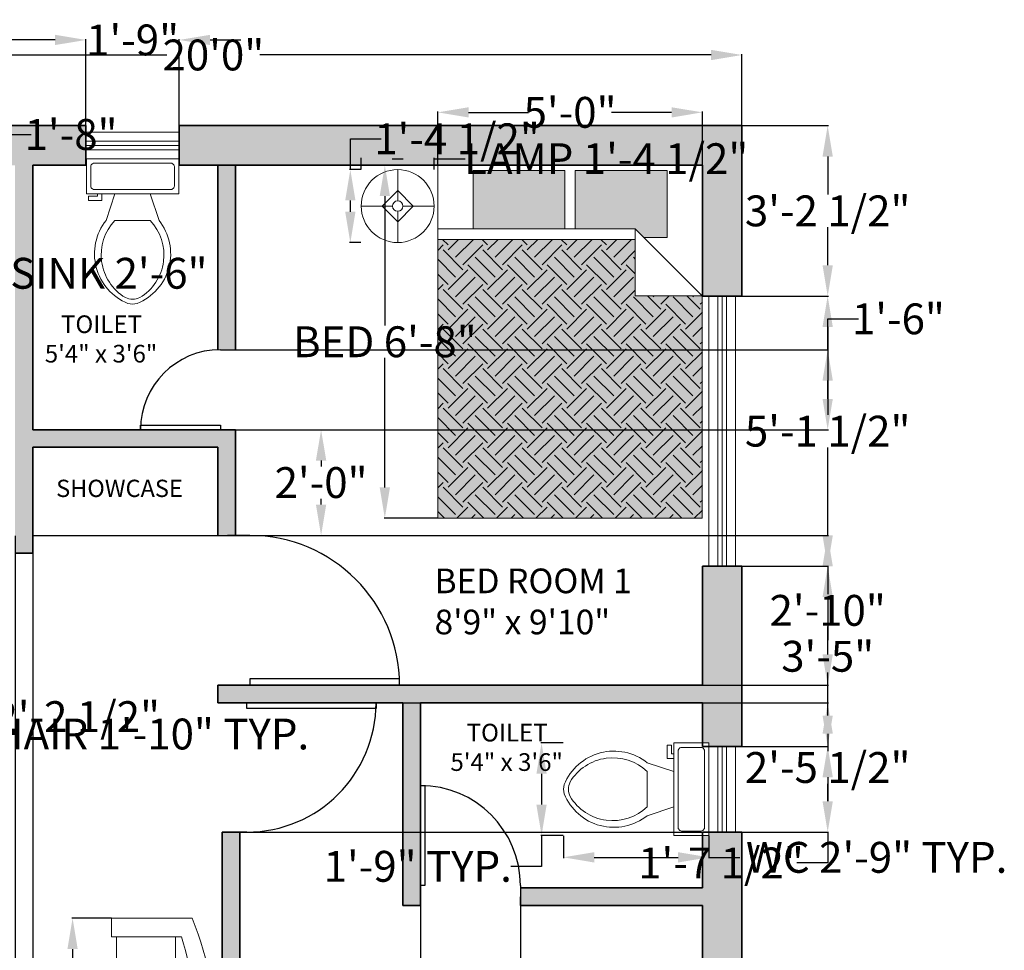
# Model space of a CAD drawing. Units: inches. Extents: x -8 to 329, y 10 to 430.
# Tile 4 of 4: x 106 to 329, y 213 to 424. Entities that reach past the tile are written whole.
import ezdxf

# ---------------------------------------------------------------- set-up
doc = ezdxf.new("R2010")
doc.units = ezdxf.units.IN
doc.header["$MEASUREMENT"] = 0
for name, color, linetype, lineweight in [('A-ANNO-DIMS', 2, 'Continuous', 18), ('A-ANNO-TEXT', 7, 'Continuous', 18), ('A-AREA-IDEN', 7, 'Continuous', 18), ('A-DOOR', 3, 'Continuous', 25), ('A-FLOR-CASE', 9, 'Continuous', 25), ('A-FLOR-FIXT', 9, 'Continuous', 18), ('A-FURN', 8, 'Continuous', 18), ('A-GLAZ', 4, 'Continuous', 18), ('A-WALL', 7, 'Continuous', 35), ('A-WALL-PATT', 253, 'Continuous', 13)]:
    doc.layers.add(name, color=color, linetype=linetype, lineweight=lineweight)
doc.layers.add('A-FURN-BASE-PATT', color=144, linetype='Continuous', lineweight=13, true_color=0x1e788f)
doc.layers.add('A-FURN-PATT', color=39, linetype='Continuous', lineweight=13, true_color=0x603913)
doc.styles.get("Standard").update_dxf_attribs({"font": 'arial.ttf'})
doc.dimstyles.get("Standard").update_dxf_attribs({"dimtxt": 7, "dimasz": 7, "dimexe": 0.18, "dimexo": 0.0625, "dimgap": 0.09, "dimtad": 0, "dimtih": 1, "dimtoh": 1, "dimdec": 0, "dimzin": 0, "dimdsep": 46, "dimlunit": 3, "dimtxsty": 'Standard', "dimcen": 0.09, "dimadec": 0, "dimazin": 0, "dimtfac": 1, "dimtdec": 0, "dimtofl": 0, "dimtmove": 0, "dimatfit": 3, "dimfxl": 1, "dimtolj": 1, "dimtzin": 0, "dimarcsym": 0})
pattern_1 = [(45, (0, 0), (0, 8.98026), [6.35, -6.35]), (45, (-1.684, 1.684), (0, 8.98026), [6.35, -6.35]), (45, (-3.3676, 3.3676), (0, 8.98026), [6.35, -6.35]), (135, (-3.3676, 4.49), (-8.98026, 0), [6.35, -6.35]), (135, (-1.684, 6.174), (-8.98026, 0), [6.35, -6.35]), (135, (0, 7.858), (-8.98026, 0), [6.35, -6.35])]

# ---------------------------------------------------------------- blocks, each defined once
blk = doc.blocks.new('Bed - Queen')
for p, q in [((0, -80.00003), (0, 0)), ((0, 0), (59.99999, 0)), ((59.99999, 0), (59.99999, -80.00003)), ((7.99999, -1.2), (28.79998, -1.2)), ((7.99999, -14.4), (7.99999, -1.2)), ((28.79998, -1.2), (28.79998, -14.4)), ((31.19999, -1.2), (51.99999, -1.2)), ((31.19999, -14.4), (31.19999, -1.2)), ((51.99999, -1.2), (51.99999, -16.4)), ((0, -14.4), (44.8, -14.4)), ((59.99999, -29.6), (44.8, -14.4)), ((44.8, -14.4), (44.8, -29.6)), ((44.8, -16.8), (0, -16.8)), ((51.99999, -16.4), (46.79936, -16.4)), ((44.8, -29.6), (59.99999, -29.6)), ((59.99999, -80.00003), (0, -80.00003))]:
    blk.add_line(p, q)
blk = doc.blocks.new('Sofa - Roundback 7 ft.')
for p, q in [((-12.00002, -32.4421), (-12.00003, -6.5971)), ((11.99997, -32.4421), (11.99998, -6.5971)), ((-36.000027, -34), (-36.000027, -11.4696)), ((35.99998, -34), (35.99998, -11.4696)), ((-35.999844, -13.3819), (35.9998, -13.3819)), ((-36.000027, -32.4421), (35.99998, -32.4421))]:
    blk.add_line(p, q)
for points in [[(-36.000027, -34), (-42.000027, -34), (-42.000027, -8)], [(41.99998, -8), (41.99998, -34), (35.99998, -34)]]:
    blk.add_lwpolyline(points)
for centre, radius, start, end in [((0, -114.25), 114.25, 68.43141, 111.5686), ((-0.00001, -127.1968), 121.1968, 72.72033, 107.2797)]:
    blk.add_arc(centre, radius, start, end)
blk = doc.blocks.new('Toilet - top')
for p, q in [((9.5, -6), (9.5, -2)), ((-10, -8.5), (-8, -8.5)), ((-10, -9.5), (-10, -8.5)), ((-8, -8.5), (-8, -8)), ((-7, -8), (-7, -9.5)), ((-4, -8), (-6, -14)), ((4, -8), (6, -14)), ((-7, -9.5), (-10, -9.5)), ((4, -14), (-4, -14))]:
    blk.add_line(p, q)
blk.add_lwpolyline([(10.5, -8), (10.5, 0), (-10.5, 0), (-10.5, -8)], close=True)
for points in [[(-9.5, -2), (-9.5, -6)], [(8.5, -1), (-8.5, -1)], [(-8.5, -7), (8.5, -7)]]:
    blk.add_lwpolyline(points)
for centre, radius, start, end in [((-8.62, -1.88), 0.884, 81.8699, 188.1301), ((8.62, -1.88), 0.884, 351.8699, 98.1301), ((-8.62, -6.12), 0.884, 171.8699, 278.1301), ((8.62, -6.12), 0.884, 261.8699, 8.1301), ((3.52, -21.58), 12.17, 141.4691, 247.9714), ((4.2, -21.82), 11.33, 136.3677, 238.9468), ((-3.52, -21.58), 12.17, 292.0284, 38.5307), ((-4.2, -21.82), 11.33, 301.053, 43.6321), ((0, -27.88), 4, 245.7318, 294.2682), ((0, -29), 4, 254.8605, 285.1395)]:
    blk.add_arc(centre, radius, start, end)
blk = doc.blocks.new('*U10')
for p, q in [((0, 0), (0, -6)), ((40, 0), (40, -6))]:
    blk.add_line(p, q)
blk.add_lwpolyline([(0, 0), (0, 40), (1.75, 40), (1.75, 0)], close=True)
blk.add_arc((0, 0), 40, 0, 90)
blk = doc.blocks.new('*U13')
for p, q in [((0, 0), (0, -6)), ((32, 0), (32, -6))]:
    blk.add_line(p, q)
blk.add_lwpolyline([(0, 0), (0, 32), (1.75, 32), (1.75, 0)], close=True)
blk.add_arc((0, 0), 32, 0, 90)
blk = doc.blocks.new('*U12')
for p, q in [((0, 0), (0, -6)), ((-40, 0), (-40, -6))]:
    blk.add_line(p, q)
blk.add_lwpolyline([(0, 0), (0, 40), (-1.75, 40), (-1.75, 0)], close=True)
blk.add_arc((0, 0), 40, 90, 180)
blk = doc.blocks.new('Lamp - Table')
for p, q in [((0, 7), (0, 1)), ((0, 3), (-3, 0)), ((3, 0), (0, 3)), ((-1, 0), (-7, 0)), ((-3, 0), (0, -3)), ((0, -3), (3, 0)), ((1, 0), (7, 0)), ((0, -1), (0, -7))]:
    blk.add_line(p, q)
for radius in [7, 1]:
    blk.add_circle((0, 0), radius)
blk = doc.blocks.new('*D16')
at = {"layer": 'A-ANNO-DIMS', "color": 0, "lineweight": -2, "transparency": 16777216}
for p, q in [((29.9, 399.83), (29.9, 415.98)), ((36.9, 415.8), (139.36, 415.8)), ((262.9, 415.8), (160.45, 415.8)), ((269.9, 399.83), (269.9, 415.98))]:
    blk.add_line(p, q, dxfattribs=at)
at = {"layer": 'A-ANNO-DIMS', "color": 0, "transparency": 16777216}
for points in [[(36.9, 416.96), (36.9, 414.63), (29.9, 415.8)], [(262.9, 416.96), (262.9, 414.63), (269.9, 415.8)]]:
    blk.add_solid(points, dxfattribs=at)
at = {"layer": 'Defpoints', "color": 0, "transparency": 16777216}
for p in [(269.9, 415.8), (29.9, 399.76), (269.9, 399.76)]:
    blk.add_point(p, dxfattribs=at)
at = {"layer": 'A-ANNO-DIMS', "color": 0, "transparency": 16777216, "insert": (149.9, 415.8), "char_height": 7, "attachment_point": 5}
blk.add_mtext('\\A1;20\'0"', dxfattribs=at)
blk = doc.blocks.new('*D18')
at = {"layer": 'A-ANNO-DIMS', "color": 0, "lineweight": -2, "transparency": 16777216}
for p, q in [((200.77, 390.76), (188.64, 390.76)), ((188.82, 383.76), (188.82, 354.38)), ((188.82, 317.68), (188.82, 347.06)), ((200.77, 310.68), (188.64, 310.68))]:
    blk.add_line(p, q, dxfattribs=at)
at = {"layer": 'A-ANNO-DIMS', "color": 0, "transparency": 16777216}
for points in [[(187.65, 383.76), (189.99, 383.76), (188.82, 390.76)], [(187.65, 317.68), (189.99, 317.68), (188.82, 310.68)]]:
    blk.add_solid(points, dxfattribs=at)
at = {"layer": 'Defpoints', "color": 0, "transparency": 16777216}
for p in [(188.82, 390.76), (200.83, 390.76), (200.83, 310.68)]:
    blk.add_point(p, dxfattribs=at)
at = {"layer": 'A-ANNO-DIMS', "color": 0, "transparency": 16777216, "insert": (188.82, 350.72), "char_height": 7, "attachment_point": 5}
blk.add_mtext('\\A1;BED 6\'-8"', dxfattribs=at)
blk = doc.blocks.new('*D19')
at = {"layer": 'A-ANNO-DIMS', "color": 0, "lineweight": -2, "transparency": 16777216}
for p, q in [((200.83, 390.83), (200.83, 402.96)), ((207.83, 402.78), (221.47, 402.78)), ((253.9, 402.78), (240.26, 402.78)), ((260.9, 390.83), (260.9, 402.96))]:
    blk.add_line(p, q, dxfattribs=at)
at = {"layer": 'A-ANNO-DIMS', "color": 0, "transparency": 16777216}
for points in [[(207.83, 403.94), (207.83, 401.61), (200.83, 402.78)], [(253.9, 403.94), (253.9, 401.61), (260.9, 402.78)]]:
    blk.add_solid(points, dxfattribs=at)
at = {"layer": 'Defpoints', "color": 0, "transparency": 16777216}
for p in [(260.9, 402.78), (200.83, 390.76), (260.9, 390.76)]:
    blk.add_point(p, dxfattribs=at)
at = {"layer": 'A-ANNO-DIMS', "color": 0, "transparency": 16777216, "insert": (230.87, 402.78), "char_height": 7, "attachment_point": 5}
blk.add_mtext('\\A1;5\'-0"', dxfattribs=at)
blk = doc.blocks.new('*D22')
at = {"layer": 'A-ANNO-DIMS', "color": 0, "lineweight": -2, "transparency": 16777216}
for p, q in [((40.19, 261.77), (40.19, 265.83)), ((47.19, 265.65), (59.46, 265.65)), ((66.46, 261.77), (66.46, 265.83)), ((66.46, 265.65), (73.46, 265.65))]:
    blk.add_line(p, q, dxfattribs=at)
at = {"layer": 'A-ANNO-DIMS', "color": 0, "transparency": 16777216}
for points in [[(47.19, 266.81), (47.19, 264.48), (40.19, 265.65)], [(59.46, 266.81), (59.46, 264.48), (66.46, 265.65)]]:
    blk.add_solid(points, dxfattribs=at)
at = {"layer": 'Defpoints', "color": 0, "transparency": 16777216}
for p in [(66.46, 265.65), (40.19, 261.71), (66.46, 261.71)]:
    blk.add_point(p, dxfattribs=at)
at = {"layer": 'A-ANNO-DIMS', "color": 0, "transparency": 16777216, "insert": (105.53, 265.65), "char_height": 7, "attachment_point": 5}
blk.add_mtext('\\A1;LAMP 2\'-2 1/2"', dxfattribs=at)
blk = doc.blocks.new('*D24')
at = {"layer": 'A-ANNO-DIMS', "color": 0, "lineweight": -2, "transparency": 16777216}
for p, q in [((183.47, 389.84), (183.47, 392.44)), ((190.47, 392.26), (193.02, 392.26)), ((200.02, 389.84), (200.02, 392.44)), ((200.02, 392.26), (207.02, 392.26))]:
    blk.add_line(p, q, dxfattribs=at)
at = {"layer": 'A-ANNO-DIMS', "color": 0, "transparency": 16777216}
for points in [[(190.47, 393.43), (190.47, 391.09), (183.47, 392.26)], [(193.02, 393.43), (193.02, 391.09), (200.02, 392.26)]]:
    blk.add_solid(points, dxfattribs=at)
at = {"layer": 'Defpoints', "color": 0, "transparency": 16777216}
for p in [(200.02, 392.26), (183.47, 389.78), (200.02, 389.78)]:
    blk.add_point(p, dxfattribs=at)
at = {"layer": 'A-ANNO-DIMS', "color": 0, "transparency": 16777216, "insert": (239.08, 392.26), "char_height": 7, "attachment_point": 5}
blk.add_mtext('\\A1;LAMP 1\'-4 1/2"', dxfattribs=at)
blk = doc.blocks.new('*D25')
at = {"layer": 'A-ANNO-DIMS', "color": 0, "lineweight": -2, "transparency": 16777216}
for p, q in [((180.99, 389.78), (180.99, 396.78)), ((180.99, 396.78), (187.99, 396.78)), ((183.41, 389.78), (180.81, 389.78)), ((180.99, 380.23), (180.99, 382.78)), ((183.41, 373.23), (180.81, 373.23))]:
    blk.add_line(p, q, dxfattribs=at)
at = {"layer": 'A-ANNO-DIMS', "color": 0, "transparency": 16777216}
for points in [[(179.82, 382.78), (182.16, 382.78), (180.99, 389.78)], [(179.82, 380.23), (182.16, 380.23), (180.99, 373.23)]]:
    blk.add_solid(points, dxfattribs=at)
at = {"layer": 'Defpoints', "color": 0, "transparency": 16777216}
for p in [(180.99, 389.78), (183.47, 389.78), (183.47, 373.23)]:
    blk.add_point(p, dxfattribs=at)
at = {"layer": 'A-ANNO-DIMS', "color": 0, "transparency": 16777216, "insert": (205.21, 396.78), "char_height": 7, "attachment_point": 5}
blk.add_mtext('\\A1;1\'-4 1/2"', dxfattribs=at)
blk = doc.blocks.new('*D28')
at = {"layer": 'A-ANNO-DIMS', "color": 0, "lineweight": -2, "transparency": 16777216}
for p, q in [((63.23, 258.5), (63.23, 261.88)), ((70.23, 261.7), (78.03, 261.7)), ((85.03, 258.5), (85.03, 261.88)), ((85.03, 261.7), (92.03, 261.7))]:
    blk.add_line(p, q, dxfattribs=at)
at = {"layer": 'A-ANNO-DIMS', "color": 0, "transparency": 16777216}
for points in [[(70.23, 262.87), (70.23, 260.54), (63.23, 261.7)], [(78.03, 262.87), (78.03, 260.54), (85.03, 261.7)]]:
    blk.add_solid(points, dxfattribs=at)
at = {"layer": 'Defpoints', "color": 0, "transparency": 16777216}
for p in [(85.03, 261.7), (63.23, 258.43), (85.03, 258.43)]:
    blk.add_point(p, dxfattribs=at)
at = {"layer": 'A-ANNO-DIMS', "color": 0, "transparency": 16777216, "insert": (132.71, 261.7), "char_height": 7, "attachment_point": 5}
blk.add_mtext('\\A1;CHAIR 1\'-10" TYP.', dxfattribs=at)
blk = doc.blocks.new('*D30')
at = {"layer": 'A-ANNO-DIMS', "color": 0, "lineweight": -2, "transparency": 16777216}
for p, q in [((229.35, 238.6), (229.35, 233.53)), ((262.4, 238.6), (262.4, 233.53)), ((236.35, 233.71), (255.4, 233.71)), ((262.4, 233.71), (269.4, 233.71))]:
    blk.add_line(p, q, dxfattribs=at)
at = {"layer": 'A-ANNO-DIMS', "color": 0, "transparency": 16777216}
for points in [[(236.35, 234.88), (236.35, 232.54), (229.35, 233.71)], [(255.4, 234.88), (255.4, 232.54), (262.4, 233.71)]]:
    blk.add_solid(points, dxfattribs=at)
at = {"layer": 'Defpoints', "color": 0, "transparency": 16777216}
for p in [(229.35, 238.67), (262.4, 238.67), (262.4, 233.71)]:
    blk.add_point(p, dxfattribs=at)
at = {"layer": 'A-ANNO-DIMS', "color": 0, "transparency": 16777216, "insert": (300.47, 233.71), "char_height": 7, "attachment_point": 5}
blk.add_mtext('\\A1;WC 2\'-9" TYP.', dxfattribs=at)
blk = doc.blocks.new('*D31')
at = {"layer": 'A-ANNO-DIMS', "color": 0, "lineweight": -2, "transparency": 16777216}
for p, q in [((229.29, 259.67), (224.22, 259.67)), ((224.4, 252.67), (224.4, 245.67)), ((229.29, 238.67), (224.22, 238.67)), ((224.4, 238.67), (224.4, 231.67)), ((224.4, 231.67), (217.4, 231.67))]:
    blk.add_line(p, q, dxfattribs=at)
at = {"layer": 'A-ANNO-DIMS', "color": 0, "transparency": 16777216}
for points in [[(223.23, 252.67), (225.56, 252.67), (224.4, 259.67)], [(223.23, 245.67), (225.56, 245.67), (224.4, 238.67)]]:
    blk.add_solid(points, dxfattribs=at)
at = {"layer": 'Defpoints', "color": 0, "transparency": 16777216}
for p in [(229.35, 259.67), (224.4, 238.67), (229.35, 238.67)]:
    blk.add_point(p, dxfattribs=at)
at = {"layer": 'A-ANNO-DIMS', "color": 0, "transparency": 16777216, "insert": (196.3, 231.67), "char_height": 7, "attachment_point": 5}
blk.add_mtext('\\A1;1\'-9" TYP.', dxfattribs=at)
blk = doc.blocks.new('*D32')
at = {"layer": 'A-ANNO-DIMS', "color": 0, "lineweight": -2, "transparency": 16777216}
for p, q in [((126.75, 219.9), (117.76, 219.9)), ((117.94, 212.9), (117.94, 194.03)), ((117.94, 167.75), (117.94, 186.61)), ((126.75, 160.75), (117.76, 160.75))]:
    blk.add_line(p, q, dxfattribs=at)
at = {"layer": 'A-ANNO-DIMS', "color": 0, "transparency": 16777216}
for points in [[(116.77, 212.9), (119.1, 212.9), (117.94, 219.9)], [(116.77, 167.75), (119.1, 167.75), (117.94, 160.75)]]:
    blk.add_solid(points, dxfattribs=at)
at = {"layer": 'Defpoints', "color": 0, "transparency": 16777216}
for p in [(126.81, 219.9), (117.94, 160.75), (126.81, 160.75)]:
    blk.add_point(p, dxfattribs=at)
at = {"layer": 'A-ANNO-DIMS', "color": 0, "transparency": 16777216, "insert": (117.94, 190.32), "char_height": 7, "attachment_point": 5}
blk.add_mtext('\\A1;SOFA 4\'-11"', dxfattribs=at)
blk = doc.blocks.new('*D40')
at = {"layer": 'A-ANNO-DIMS', "color": 0, "lineweight": -2, "transparency": 16777216}
for p, q in [((67.02, 370.7), (67.02, 366.08)), ((97.02, 370.7), (97.02, 366.08)), ((74.02, 366.26), (90.02, 366.26)), ((97.02, 366.26), (104.02, 366.26))]:
    blk.add_line(p, q, dxfattribs=at)
at = {"layer": 'A-ANNO-DIMS', "color": 0, "transparency": 16777216}
for points in [[(74.02, 367.43), (74.02, 365.1), (67.02, 366.26)], [(90.02, 367.43), (90.02, 365.1), (97.02, 366.26)]]:
    blk.add_solid(points, dxfattribs=at)
at = {"layer": 'Defpoints', "color": 0, "transparency": 16777216}
for p in [(67.02, 370.76), (97.02, 370.76), (97.02, 366.26)]:
    blk.add_point(p, dxfattribs=at)
at = {"layer": 'A-ANNO-DIMS', "color": 0, "transparency": 16777216, "insert": (126.17, 366.26), "char_height": 7, "attachment_point": 5}
blk.add_mtext('\\A1;SINK 2\'-6"', dxfattribs=at)
blk = doc.blocks.new('*D41')
at = {"layer": 'A-ANNO-DIMS', "color": 0, "lineweight": -2, "transparency": 16777216}
for p, q in [((101.52, 390.76), (101.52, 397.76)), ((101.52, 397.76), (108.52, 397.76)), ((97.09, 390.76), (101.7, 390.76)), ((101.52, 377.76), (101.52, 383.76)), ((97.09, 370.76), (101.7, 370.76))]:
    blk.add_line(p, q, dxfattribs=at)
at = {"layer": 'A-ANNO-DIMS', "color": 0, "transparency": 16777216}
for points in [[(100.36, 383.76), (102.69, 383.76), (101.52, 390.76)], [(100.36, 377.76), (102.69, 377.76), (101.52, 370.76)]]:
    blk.add_solid(points, dxfattribs=at)
at = {"layer": 'Defpoints', "color": 0, "transparency": 16777216}
for p in [(97.02, 390.76), (101.52, 390.76), (97.02, 370.76)]:
    blk.add_point(p, dxfattribs=at)
at = {"layer": 'A-ANNO-DIMS', "color": 0, "transparency": 16777216, "insert": (117.59, 397.76), "char_height": 7, "attachment_point": 5}
blk.add_mtext('\\A1;1\'-8"', dxfattribs=at)
blk = doc.blocks.new('*D42')
at = {"layer": 'A-ANNO-DIMS', "color": 0, "lineweight": -2, "transparency": 16777216}
for p, q in [((150.96, 306.76), (289.53, 306.76)), ((289.35, 299.76), (289.35, 293.43)), ((289.35, 279.76), (289.35, 286.1)), ((150.96, 272.76), (289.53, 272.76))]:
    blk.add_line(p, q, dxfattribs=at)
at = {"layer": 'A-ANNO-DIMS', "color": 0, "transparency": 16777216}
for points in [[(288.18, 299.76), (290.52, 299.76), (289.35, 306.76)], [(288.18, 279.76), (290.52, 279.76), (289.35, 272.76)]]:
    blk.add_solid(points, dxfattribs=at)
at = {"layer": 'Defpoints', "color": 0, "transparency": 16777216}
for p in [(150.9, 306.76), (289.35, 306.76), (150.9, 272.76)]:
    blk.add_point(p, dxfattribs=at)
at = {"layer": 'A-ANNO-DIMS', "color": 0, "transparency": 16777216, "insert": (289.35, 289.76), "char_height": 7, "attachment_point": 5}
blk.add_mtext('\\A1;2\'-10"', dxfattribs=at)
blk = doc.blocks.new('*D43')
at = {"layer": 'A-ANNO-DIMS', "color": 0, "lineweight": -2, "transparency": 16777216}
for p, q in [((150.96, 268.76), (289.53, 268.76)), ((289.35, 261.76), (289.35, 257.81)), ((289.35, 246.44), (289.35, 250.39)), ((151.96, 239.44), (289.53, 239.44))]:
    blk.add_line(p, q, dxfattribs=at)
at = {"layer": 'A-ANNO-DIMS', "color": 0, "transparency": 16777216}
for points in [[(288.18, 261.76), (290.52, 261.76), (289.35, 268.76)], [(288.18, 246.44), (290.52, 246.44), (289.35, 239.44)]]:
    blk.add_solid(points, dxfattribs=at)
at = {"layer": 'Defpoints', "color": 0, "transparency": 16777216}
for p in [(150.9, 268.76), (151.9, 239.44), (289.35, 239.44)]:
    blk.add_point(p, dxfattribs=at)
at = {"layer": 'A-ANNO-DIMS', "color": 0, "transparency": 16777216, "insert": (289.35, 254.1), "char_height": 7, "attachment_point": 5}
blk.add_mtext('\\A1;2\'-5 1/2"', dxfattribs=at)
blk = doc.blocks.new('*D47')
at = {"layer": 'A-ANNO-DIMS', "color": 0, "lineweight": -2, "transparency": 16777216}
for p, q in [((289.35, 348.92), (289.35, 355.92)), ((289.35, 355.92), (296.35, 355.92)), ((154.96, 348.92), (289.53, 348.92)), ((289.35, 337.76), (289.35, 341.92)), ((154.96, 330.76), (289.53, 330.76))]:
    blk.add_line(p, q, dxfattribs=at)
at = {"layer": 'A-ANNO-DIMS', "color": 0, "transparency": 16777216}
for points in [[(288.18, 341.92), (290.52, 341.92), (289.35, 348.92)], [(288.18, 337.76), (290.52, 337.76), (289.35, 330.76)]]:
    blk.add_solid(points, dxfattribs=at)
at = {"layer": 'Defpoints', "color": 0, "transparency": 16777216}
for p in [(154.9, 348.92), (289.35, 348.92), (154.9, 330.76)]:
    blk.add_point(p, dxfattribs=at)
at = {"layer": 'A-ANNO-DIMS', "color": 0, "transparency": 16777216, "insert": (305.41, 355.92), "char_height": 7, "attachment_point": 5}
blk.add_mtext('\\A1;1\'-6"', dxfattribs=at)
blk = doc.blocks.new('*D48')
at = {"layer": 'A-ANNO-DIMS', "color": 0, "lineweight": -2, "transparency": 16777216}
for p, q in [((196.9, 226.25), (196.9, 20.13)), ((219.6, 226.7), (219.6, 20.13)), ((203.9, 20.31), (212.6, 20.31)), ((219.6, 20.31), (226.6, 20.31))]:
    blk.add_line(p, q, dxfattribs=at)
at = {"layer": 'A-ANNO-DIMS', "color": 0, "transparency": 16777216}
for points in [[(203.9, 21.48), (203.9, 19.15), (196.9, 20.31)], [(212.6, 21.48), (212.6, 19.15), (219.6, 20.31)]]:
    blk.add_solid(points, dxfattribs=at)
at = {"layer": 'Defpoints', "color": 0, "transparency": 16777216}
for p in [(196.9, 226.31), (219.6, 226.76), (219.6, 20.31)]:
    blk.add_point(p, dxfattribs=at)
at = {"layer": 'A-ANNO-DIMS', "color": 0, "transparency": 16777216, "insert": (246.54, 20.31), "char_height": 7, "attachment_point": 5}
blk.add_mtext('\\A1;1\'-10 1/2"', dxfattribs=at)
blk = doc.blocks.new('*D49')
at = {"layer": 'A-ANNO-DIMS', "color": 0, "lineweight": -2, "transparency": 16777216}
for p, q in [((154.96, 330.76), (174.53, 330.76)), ((174.35, 323.76), (174.35, 322.43)), ((174.35, 313.76), (174.35, 315.1)), ((154.96, 306.76), (174.53, 306.76))]:
    blk.add_line(p, q, dxfattribs=at)
at = {"layer": 'A-ANNO-DIMS', "color": 0, "transparency": 16777216}
for points in [[(173.18, 323.76), (175.52, 323.76), (174.35, 330.76)], [(173.18, 313.76), (175.52, 313.76), (174.35, 306.76)]]:
    blk.add_solid(points, dxfattribs=at)
at = {"layer": 'Defpoints', "color": 0, "transparency": 16777216}
for p in [(154.9, 330.76), (154.9, 306.76), (174.35, 306.76)]:
    blk.add_point(p, dxfattribs=at)
at = {"layer": 'A-ANNO-DIMS', "color": 0, "transparency": 16777216, "insert": (174.35, 318.76), "char_height": 7, "attachment_point": 5}
blk.add_mtext('\\A1;2\'-0"', dxfattribs=at)
blk = doc.blocks.new('*D50')
at = {"layer": 'A-ANNO-DIMS', "color": 0, "lineweight": -2, "transparency": 16777216}
for p, q in [((78.68, 302.7), (78.68, 20.13)), ((104.9, 302.7), (104.9, 20.13)), ((71.68, 20.31), (64.68, 20.31)), ((111.9, 20.31), (118.9, 20.31))]:
    blk.add_line(p, q, dxfattribs=at)
at = {"layer": 'A-ANNO-DIMS', "color": 0, "transparency": 16777216}
for points in [[(71.68, 21.48), (71.68, 19.15), (78.68, 20.31)], [(111.9, 21.48), (111.9, 19.15), (104.9, 20.31)]]:
    blk.add_solid(points, dxfattribs=at)
at = {"layer": 'Defpoints', "color": 0, "transparency": 16777216}
for p in [(78.68, 302.76), (104.9, 302.76), (104.9, 20.31)]:
    blk.add_point(p, dxfattribs=at)
at = {"layer": 'A-ANNO-DIMS', "color": 0, "transparency": 16777216, "insert": (91.79, 20.31), "char_height": 7, "attachment_point": 5}
blk.add_mtext('\\A1;2\'-2"', dxfattribs=at)
blk = doc.blocks.new('*D55')
at = {"layer": 'A-ANNO-DIMS', "color": 0, "lineweight": -2, "transparency": 16777216}
for p, q in [((269.96, 361.08), (289.53, 361.08)), ((289.35, 354.08), (289.35, 334.14)), ((289.35, 306.78), (289.35, 326.72)), ((269.96, 299.78), (289.53, 299.78))]:
    blk.add_line(p, q, dxfattribs=at)
at = {"layer": 'A-ANNO-DIMS', "color": 0, "transparency": 16777216}
for points in [[(288.18, 354.08), (290.52, 354.08), (289.35, 361.08)], [(288.18, 306.78), (290.52, 306.78), (289.35, 299.78)]]:
    blk.add_solid(points, dxfattribs=at)
at = {"layer": 'Defpoints', "color": 0, "transparency": 16777216}
for p in [(269.9, 361.08), (269.9, 299.78), (289.35, 299.78)]:
    blk.add_point(p, dxfattribs=at)
at = {"layer": 'A-ANNO-DIMS', "color": 0, "transparency": 16777216, "insert": (289.35, 330.43), "char_height": 7, "attachment_point": 5}
blk.add_mtext('\\A1;5\'-1 1/2"', dxfattribs=at)
blk = doc.blocks.new('*D56')
at = {"layer": 'A-ANNO-DIMS', "color": 0, "lineweight": -2, "transparency": 16777216}
for p, q in [((269.96, 258.9), (289.53, 258.9)), ((289.35, 251.9), (289.35, 246.44)), ((269.96, 239.44), (289.53, 239.44)), ((289.35, 239.44), (289.35, 232.44)), ((289.35, 232.44), (282.35, 232.44))]:
    blk.add_line(p, q, dxfattribs=at)
at = {"layer": 'A-ANNO-DIMS', "color": 0, "transparency": 16777216}
for points in [[(288.18, 251.9), (290.52, 251.9), (289.35, 258.9)], [(288.18, 246.44), (290.52, 246.44), (289.35, 239.44)]]:
    blk.add_solid(points, dxfattribs=at)
at = {"layer": 'Defpoints', "color": 0, "transparency": 16777216}
for p in [(269.9, 258.9), (269.9, 239.44), (289.35, 239.44)]:
    blk.add_point(p, dxfattribs=at)
at = {"layer": 'A-ANNO-DIMS', "color": 0, "transparency": 16777216, "insert": (265.13, 232.44), "char_height": 7, "attachment_point": 5}
blk.add_mtext('\\A1;1\'-7 1/2"', dxfattribs=at)
blk = doc.blocks.new('*D58')
at = {"layer": 'A-ANNO-DIMS', "color": 0, "lineweight": -2, "transparency": 16777216}
for p, q in [((113.96, 419.21), (106.96, 419.21)), ((120.96, 399.83), (120.96, 419.39)), ((142.16, 399.83), (142.16, 419.39)), ((149.16, 419.21), (156.16, 419.21))]:
    blk.add_line(p, q, dxfattribs=at)
at = {"layer": 'A-ANNO-DIMS', "color": 0, "transparency": 16777216}
for points in [[(113.96, 420.38), (113.96, 418.05), (120.96, 419.21)], [(149.16, 420.38), (149.16, 418.05), (142.16, 419.21)]]:
    blk.add_solid(points, dxfattribs=at)
at = {"layer": 'Defpoints', "color": 0, "transparency": 16777216}
for p in [(142.16, 419.21), (120.96, 399.76), (142.16, 399.76)]:
    blk.add_point(p, dxfattribs=at)
at = {"layer": 'A-ANNO-DIMS', "color": 0, "transparency": 16777216, "insert": (131.56, 419.21), "char_height": 7, "attachment_point": 5}
blk.add_mtext('\\A1;1\'-9"', dxfattribs=at)
blk = doc.blocks.new('*D62')
at = {"layer": 'A-ANNO-DIMS', "color": 0, "lineweight": -2, "transparency": 16777216}
for p, q in [((269.96, 399.76), (289.53, 399.76)), ((289.35, 392.76), (289.35, 384.14)), ((289.35, 368.08), (289.35, 376.71)), ((269.96, 361.08), (289.53, 361.08))]:
    blk.add_line(p, q, dxfattribs=at)
at = {"layer": 'A-ANNO-DIMS', "color": 0, "transparency": 16777216}
for points in [[(288.18, 392.76), (290.52, 392.76), (289.35, 399.76)], [(288.18, 368.08), (290.52, 368.08), (289.35, 361.08)]]:
    blk.add_solid(points, dxfattribs=at)
at = {"layer": 'Defpoints', "color": 0, "transparency": 16777216}
for p in [(269.9, 399.76), (269.9, 361.08), (289.35, 361.08)]:
    blk.add_point(p, dxfattribs=at)
at = {"layer": 'A-ANNO-DIMS', "color": 0, "transparency": 16777216, "insert": (289.35, 380.42), "char_height": 7, "attachment_point": 5}
blk.add_mtext('\\A1;3\'-2 1/2"', dxfattribs=at)
blk = doc.blocks.new('*D63')
at = {"layer": 'A-ANNO-DIMS', "color": 0, "lineweight": -2, "transparency": 16777216}
for p, q in [((269.96, 299.78), (289.53, 299.78)), ((289.35, 292.78), (289.35, 283)), ((289.35, 265.9), (289.35, 275.67)), ((269.96, 258.9), (289.53, 258.9))]:
    blk.add_line(p, q, dxfattribs=at)
at = {"layer": 'A-ANNO-DIMS', "color": 0, "transparency": 16777216}
for points in [[(288.18, 292.78), (290.52, 292.78), (289.35, 299.78)], [(288.18, 265.9), (290.52, 265.9), (289.35, 258.9)]]:
    blk.add_solid(points, dxfattribs=at)
at = {"layer": 'Defpoints', "color": 0, "transparency": 16777216}
for p in [(269.9, 299.78), (269.9, 258.9), (289.35, 258.9)]:
    blk.add_point(p, dxfattribs=at)
at = {"layer": 'A-ANNO-DIMS', "color": 0, "transparency": 16777216, "insert": (289.35, 279.34), "char_height": 7, "attachment_point": 5}
blk.add_mtext('\\A1;3\'-5"', dxfattribs=at)
blk = doc.blocks.new('*D65')
at = {"layer": 'A-ANNO-DIMS', "color": 0, "lineweight": -2, "transparency": 16777216}
for p, q in [((29.9, 399.83), (29.9, 419.39)), ((36.9, 419.21), (66.07, 419.21)), ((113.96, 419.21), (84.8, 419.21)), ((120.96, 399.83), (120.96, 419.39))]:
    blk.add_line(p, q, dxfattribs=at)
at = {"layer": 'A-ANNO-DIMS', "color": 0, "transparency": 16777216}
for points in [[(36.9, 420.38), (36.9, 418.05), (29.9, 419.21)], [(113.96, 420.38), (113.96, 418.05), (120.96, 419.21)]]:
    blk.add_solid(points, dxfattribs=at)
at = {"layer": 'Defpoints', "color": 0, "transparency": 16777216}
for p in [(120.96, 419.21), (29.9, 399.76), (120.96, 399.76)]:
    blk.add_point(p, dxfattribs=at)
at = {"layer": 'A-ANNO-DIMS', "color": 0, "transparency": 16777216, "insert": (75.43, 419.21), "char_height": 7, "attachment_point": 5}
blk.add_mtext('\\A1;7\'-7"', dxfattribs=at)
blk = doc.blocks.new('*D70')
at = {"layer": 'A-ANNO-DIMS', "color": 0, "lineweight": -2, "transparency": 16777216}
for p, q in [((104.9, 306.7), (104.9, 20.13)), ((108.9, 306.7), (108.9, 20.13)), ((97.9, 20.31), (90.9, 20.31)), ((115.9, 20.31), (122.9, 20.31))]:
    blk.add_line(p, q, dxfattribs=at)
at = {"layer": 'A-ANNO-DIMS', "color": 0, "transparency": 16777216}
for points in [[(97.9, 21.48), (97.9, 19.15), (104.9, 20.31)], [(115.9, 21.48), (115.9, 19.15), (108.9, 20.31)]]:
    blk.add_solid(points, dxfattribs=at)
at = {"layer": 'Defpoints', "color": 0, "transparency": 16777216}
for p in [(104.9, 306.76), (108.9, 306.76), (108.9, 20.31)]:
    blk.add_point(p, dxfattribs=at)
at = {"layer": 'A-ANNO-DIMS', "color": 0, "transparency": 16777216, "insert": (132.29, 20.31), "char_height": 7, "attachment_point": 5}
blk.add_mtext('\\A1;0\'-4"', dxfattribs=at)

msp = doc.modelspace()

# ---------------------------------------------------------------- hatches: boundary and pattern name
at = {"layer": 'A-FURN-BASE-PATT'}
h = msp.add_hatch(color=256, dxfattribs=at)
h.dxf.hatch_style = 1
h.paths.add_polyline_path([(229.67, 376.35), (229.67, 389.56), (208.84, 389.56), (208.84, 376.35)])
h = msp.add_hatch(color=256, dxfattribs=at)
h.dxf.hatch_style = 1
h.paths.add_polyline_path([(245.68, 376.35), (247.69, 374.35), (252.89, 374.35), (252.89, 389.56), (232.07, 389.56), (232.07, 376.35)])
h = msp.add_hatch(color=256, dxfattribs=at)
h.dxf.hatch_style = 1
h.paths.add_polyline_path([(260.9, 310.68), (260.9, 361.13), (245.68, 361.13), (245.68, 373.94), (200.83, 373.94), (200.83, 310.68)])
at = {"layer": 'A-FURN-PATT'}
h = msp.add_hatch(dxfattribs=at)
h.set_pattern_fill('EARTH', color=256, angle=45)
h.set_pattern_definition(pattern_1)
h.paths.add_polyline_path([(260.9, 310.68), (260.9, 361.13), (245.68, 361.13), (245.68, 373.94), (200.83, 373.94), (200.83, 310.68)])
h = msp.add_hatch(dxfattribs=at)
h.set_pattern_fill('EARTH', color=256, angle=45)
h.set_pattern_definition(pattern_1)
h.paths.add_polyline_path([(260.9, 310.68), (260.9, 361.13), (245.68, 361.13), (245.68, 373.94), (200.83, 373.94), (200.83, 310.68)])
at = {"layer": 'A-WALL-PATT'}
h = msp.add_hatch(color=256, dxfattribs=at)
h.dxf.hatch_style = 1
h.paths.add_polyline_path([(29.9, 362.26), (38.9, 362.26), (38.9, 390.76), (104.9, 390.76), (104.9, 306.76), (104.9, 302.76), (108.9, 302.76), (108.9, 326.76), (150.9, 326.76), (150.9, 306.76), (154.9, 306.76), (154.9, 330.76), (151.5, 330.76), (133.34, 330.76), (108.9, 330.76), (108.9, 390.76), (120.96, 390.76), (120.96, 399.76), (29.9, 399.76)])
h = msp.add_hatch(color=256, dxfattribs=at)
h.dxf.hatch_style = 1
h.paths.add_polyline_path([(260.9, 390.76), (260.9, 361.08), (269.9, 361.08), (269.9, 399.76), (142.16, 399.76), (142.16, 390.76)])
h = msp.add_hatch(color=256, dxfattribs=at)
h.dxf.hatch_style = 1
h.paths.add_polyline_path([(154.9, 390.76), (150.9, 390.76), (150.9, 353.45), (150.9, 348.91, -0.008198), (151.5, 348.92), (154.9, 348.92), (154.9, 353.46)])
h = msp.add_hatch(color=256, dxfattribs=at)
h.dxf.hatch_style = 1
h.paths.add_polyline_path([(192.9, 222.76), (196.9, 222.76), (196.9, 268.76), (260.9, 268.76), (260.9, 259.67), (262.4, 259.67), (262.4, 258.9), (269.9, 258.9), (269.9, 299.78), (260.9, 299.78), (260.9, 272.76), (150.9, 272.76), (150.9, 268.76), (192.9, 268.76)])
h = msp.add_hatch(color=256, dxfattribs=at)
h.dxf.hatch_style = 1
h.paths.add_polyline_path([(146.32, 48.76), (146.32, 39.76), (269.9, 39.76), (269.9, 145.31), (260.9, 145.31), (260.9, 112.76), (186.22, 112.76), (155.9, 112.76), (155.9, 222.76), (155.9, 239.44), (153.1, 239.44), (151.9, 239.44), (151.9, 222.76), (151.9, 108.76), (260.9, 108.76), (260.9, 48.76)])
h = msp.add_hatch(color=256, dxfattribs=at)
h.dxf.hatch_style = 1
h.paths.add_polyline_path([(269.9, 239.44), (262.4, 239.44), (262.4, 238.67), (260.9, 238.67), (260.9, 226.76), (219.6, 226.76), (219.6, 223.9), (219.6, 222.76), (260.9, 222.76), (260.9, 195.02), (269.9, 195.02)])

# ---------------------------------------------------------------- linework, layer by layer
at = {"layer": 'A-FLOR-CASE'}
msp.add_line((108.9, 306.76), (154.9, 306.76), dxfattribs=at)
at = {"layer": 'A-GLAZ'}
for p, q in [((120.96, 398.26), (142.16, 398.26)), ((120.96, 396.26), (142.16, 396.26)), ((120.96, 395.26), (142.16, 395.26)), ((120.96, 394.26), (142.16, 394.26)), ((120.96, 392.26), (142.16, 392.26)), ((262.4, 299.78), (262.4, 361.08)), ((264.4, 299.78), (264.4, 361.08)), ((265.4, 299.78), (265.4, 361.08)), ((266.4, 299.78), (266.4, 361.08)), ((268.4, 299.78), (268.4, 361.08)), ((262.4, 258.9), (262.4, 239.44)), ((264.4, 258.9), (264.4, 239.44)), ((265.4, 258.9), (265.4, 239.44)), ((266.4, 258.9), (266.4, 239.44)), ((268.4, 258.9), (268.4, 239.44))]:
    msp.add_line(p, q, dxfattribs=at)
at = {"layer": 'A-WALL'}
for p, q in [((29.9, 399.76), (120.96, 399.76)), ((120.96, 390.76), (120.96, 399.76)), ((142.16, 390.76), (142.16, 399.76)), ((142.16, 399.76), (269.9, 399.76)), ((269.9, 399.76), (269.9, 361.08)), ((108.9, 390.76), (120.96, 390.76)), ((108.9, 330.76), (108.9, 390.76)), ((142.16, 390.76), (260.9, 390.76)), ((142.16, 390.76), (150.9, 390.76)), ((150.9, 353.45), (150.9, 390.76)), ((154.9, 353.46), (154.9, 390.76)), ((260.9, 390.76), (260.9, 361.08)), ((260.9, 361.08), (269.9, 361.08)), ((150.9, 353.45), (150.9, 348.91)), ((154.9, 353.46), (154.9, 348.92)), ((108.9, 330.76), (154.9, 330.76)), ((154.9, 306.76), (154.9, 330.76)), ((108.9, 326.76), (150.9, 326.76)), ((108.9, 302.76), (108.9, 326.76)), ((150.9, 306.76), (150.9, 326.76)), ((104.9, 302.76), (108.9, 302.76)), ((260.9, 299.78), (269.9, 299.78)), ((260.9, 299.78), (260.9, 272.76)), ((269.9, 299.78), (269.9, 258.9)), ((150.9, 268.76), (150.9, 272.76)), ((150.9, 272.76), (260.9, 272.76)), ((150.9, 268.76), (192.9, 268.76)), ((192.9, 268.76), (192.9, 222.76)), ((196.9, 268.76), (196.9, 222.76)), ((196.9, 268.76), (260.9, 268.76)), ((260.9, 268.76), (260.9, 258.9)), ((260.9, 258.9), (269.9, 258.9)), ((151.9, 222.76), (151.9, 239.44)), ((153.1, 239.44), (151.9, 239.44)), ((155.9, 222.76), (155.9, 239.45)), ((260.9, 239.44), (269.9, 239.44)), ((260.9, 239.44), (260.9, 226.76)), ((269.9, 239.44), (269.9, 195.02)), ((219.6, 226.76), (260.9, 226.76)), ((219.6, 224.76), (219.6, 222.76)), ((151.9, 222.76), (151.9, 108.76)), ((155.9, 222.76), (155.9, 112.76)), ((192.9, 222.76), (196.9, 222.76)), ((219.6, 222.76), (260.9, 222.76)), ((260.9, 222.76), (260.9, 195.02))]:
    msp.add_line(p, q, dxfattribs=at)

# ---------------------------------------------------------------- block references
at = {"layer": 'A-DOOR'}
for name, p, xscale, yscale, zscale, rotation in [('*U13', (151.5, 330.76), 0.567444325510916, 0.567444325510916, 0.567444325510916, 90), ('*U12', (158.2, 272.76), 0.8497061074006313, 0.8497061074006313, 0.8497061074006313, 270), ('*U10', (157.5, 268.76), 0.733044558001341, 0.733044558001341, 0.733044558001341, 270)]:
    msp.add_blockref(name, p, dxfattribs=dict(at, xscale=xscale, yscale=yscale, zscale=zscale, rotation=rotation))
at = {"layer": 'A-DOOR', "xscale": 0.567444325510916, "yscale": 0.567444325510916, "zscale": 0.567444325510916}
msp.add_blockref('*U10', (196.9, 227.3), dxfattribs=at)
at = {"layer": 'A-FLOR-FIXT'}
msp.add_blockref('Toilet - top', (131.56, 392.26), dxfattribs=at)
at = {"layer": 'A-FLOR-FIXT', "rotation": 270}
msp.add_blockref('Toilet - top', (262.4, 249.17), dxfattribs=at)
at = {"layer": 'A-FURN'}
for name, p, xscale, yscale, zscale in [('Lamp - Table', (191.74, 381.51), 1.181728893821856, 1.181728893821856, 1.181728893821856), ('Bed - Queen', (200.83, 390.76), 1.001099935779881, 1.001099935779881, 1.001099935779881)]:
    msp.add_blockref(name, p, dxfattribs=dict(at, xscale=xscale, yscale=yscale, zscale=zscale))
at = {"layer": 'A-FURN', "xscale": 0.704182813737638, "yscale": 0.704182813737638, "zscale": 0.704182813737638, "rotation": 270}
msp.add_blockref('Sofa - Roundback 7 ft.', (150.75, 190.32), dxfattribs=at)

# ---------------------------------------------------------------- texts
at = {"layer": 'A-ANNO-TEXT', "insert": (114.21, 319.41), "char_height": 3.921, "attachment_point": 1}
msp.add_mtext_dynamic_manual_height_columns('SHOWCASE', width=365.4317, gutter_width=19.61, heights=[5.05], dxfattribs=at)
at = {"layer": 'A-AREA-IDEN', "attachment_point": 1}
for s, width, gutter_width, insert, char_height in [('   TOILET\\P5\'4" x 3\'6"', 118.1004, 20.04, (111.63, 356.7), 4.0088), ('BED ROOM 1\\P8\'9" x 9\'10"', 164.8422, 27.98, (200.1, 299.25), 5.5954), ('   TOILET\\P5\'4" x 3\'6"', 118.1004, 20.04, (203.71, 264.02), 4.0088)]:
    msp.add_mtext_dynamic_manual_height_columns(s, width=width, gutter_width=gutter_width, heights=[0], dxfattribs=dict(at, insert=insert, char_height=char_height))

# ---------------------------------------------------------------- dimensions: what is measured, and where the dimension line sits
at = {"layer": 'A-ANNO-DIMS'}
for base, p1, p2, picture, middle in [((120.96, 419.21), (29.9, 399.76), (120.96, 399.76), '*D65', (75.43, 419.21)), ((142.16, 419.21), (120.96, 399.76), (142.16, 399.76), '*D58', (131.56, 419.21)), ((260.9, 402.78), (200.83, 390.76), (260.9, 390.76), '*D19', (230.87, 402.78)), ((108.9, 20.31), (104.9, 306.76), (108.9, 306.76), '*D70', (132.29, 20.31)), ((104.9, 20.31), (78.68, 302.76), (104.9, 302.76), '*D50', (91.79, 20.31)), ((219.6, 20.31), (196.9, 226.31), (219.6, 226.76), '*D48', (246.54, 20.31))]:
    dim = msp.add_linear_dim(base=base, p1=p1, p2=p2, dimstyle='Standard', override={"dimdec": 1, "dimlfac": 1, "dimrnd": 0, "dimzin": 1, "dimdsep": 46, "dimlunit": 4, "dimfrac": 2}, dxfattribs=at)
    dim.commit()
    dim.dimension.update_dxf_attribs({"geometry": picture, "text_midpoint": middle})
for base, p1, p2, text, override, picture, middle in [((269.9, 415.8), (29.9, 399.76), (269.9, 399.76), '<>0"', {"dimclrd": 0, "dimclre": 0, "dimclrt": 0}, '*D16', (149.9, 415.8)), ((200.0151, 392.2594), (183.4709, 389.7778), (200.0151, 389.7778), 'LAMP <>', {"dimdec": 1, "dimlfac": 1, "dimrnd": 0, "dimzin": 1, "dimdsep": 46, "dimlunit": 4, "dimfrac": 2}, '*D24', (239.0826, 392.2594)), ((97.02, 366.26), (67.02, 370.76), (97.02, 370.76), 'SINK <>', {"dimdec": 1, "dimlfac": 1, "dimrnd": 0, "dimzin": 1, "dimdsep": 46, "dimlunit": 4, "dimfrac": 2}, '*D40', (126.17, 366.26)), ((66.46, 265.65), (40.19, 261.71), (66.46, 261.71), 'LAMP <>', {"dimdec": 1, "dimlfac": 1, "dimrnd": 0, "dimzin": 1, "dimdsep": 46, "dimlunit": 4, "dimfrac": 2}, '*D22', (105.53, 265.65)), ((85.03, 261.7), (63.23, 258.43), (85.03, 258.43), 'CHAIR <> TYP.', {"dimdec": 1, "dimlfac": 1, "dimrnd": 0, "dimzin": 1, "dimdsep": 46, "dimlunit": 4, "dimfrac": 2}, '*D28', (132.71, 261.7)), ((262.4006, 233.7105), (229.3543, 238.6674), (262.4006, 238.6674), 'WC <> TYP.', {"dimdec": 1, "dimlfac": 1, "dimrnd": 0, "dimzin": 1, "dimdsep": 46, "dimlunit": 4, "dimfrac": 2}, '*D30', (300.4725, 233.7105))]:
    dim = msp.add_linear_dim(base=base, p1=p1, p2=p2, text=text, dimstyle='Standard', override=override, dxfattribs=at)
    dim.commit()
    dim.dimension.update_dxf_attribs({"geometry": picture, "text_midpoint": middle})
for base, p1, p2, angle, picture, middle in [((180.9892, 389.7778), (183.4709, 373.2336), (183.4709, 389.7778), 90, '*D25', (205.2092, 396.7778)), ((101.52, 390.76), (97.02, 370.76), (97.02, 390.76), 90, '*D41', (117.59, 397.76)), ((289.35, 361.08), (269.9, 399.76), (269.9, 361.08), 90, '*D62', (289.35, 380.42)), ((289.35, 348.92), (154.9, 330.76), (154.9, 348.92), 90, '*D47', (305.41, 355.92)), ((289.35, 299.78), (269.9, 361.08), (269.9, 299.78), 90, '*D55', (289.35, 330.43)), ((174.35, 306.76), (154.9, 330.76), (154.9, 306.76), 270, '*D49', (174.35, 318.76)), ((289.35, 306.76), (150.9, 272.76), (150.9, 306.76), 90, '*D42', (289.35, 289.76)), ((289.35, 258.9), (269.9, 299.78), (269.9, 258.9), 90, '*D63', (289.35, 279.34)), ((289.35, 239.44), (150.9, 268.76), (151.9, 239.44), 90, '*D43', (289.35, 254.1)), ((289.35, 239.44), (269.9, 258.9), (269.9, 239.44), 90, '*D56', (265.13, 232.44))]:
    dim = msp.add_linear_dim(base=base, p1=p1, p2=p2, angle=angle, dimstyle='Standard', override={"dimdec": 1, "dimlfac": 1, "dimrnd": 0, "dimzin": 1, "dimdsep": 46, "dimlunit": 4, "dimfrac": 2}, dxfattribs=at)
    dim.commit()
    dim.dimension.update_dxf_attribs({"geometry": picture, "text_midpoint": middle})
for base, p1, p2, angle, text, picture, middle in [((188.82, 390.76), (200.83, 310.68), (200.83, 390.76), 90, 'BED <>', '*D18', (188.82, 350.72)), ((224.4, 238.67), (229.35, 259.67), (229.35, 238.67), 270, '<> TYP.', '*D31', (196.3, 231.67)), ((117.9359, 160.747), (126.8086, 219.8983), (126.8086, 160.747), 270, 'SOFA <>', '*D32', (117.9359, 190.3227))]:
    dim = msp.add_linear_dim(base=base, p1=p1, p2=p2, angle=angle, text=text, dimstyle='Standard', override={"dimdec": 1, "dimlfac": 1, "dimrnd": 0, "dimzin": 1, "dimdsep": 46, "dimlunit": 4, "dimfrac": 2}, dxfattribs=at)
    dim.commit()
    dim.dimension.update_dxf_attribs({"geometry": picture, "text_midpoint": middle})

doc.saveas('drawing.dxf')
